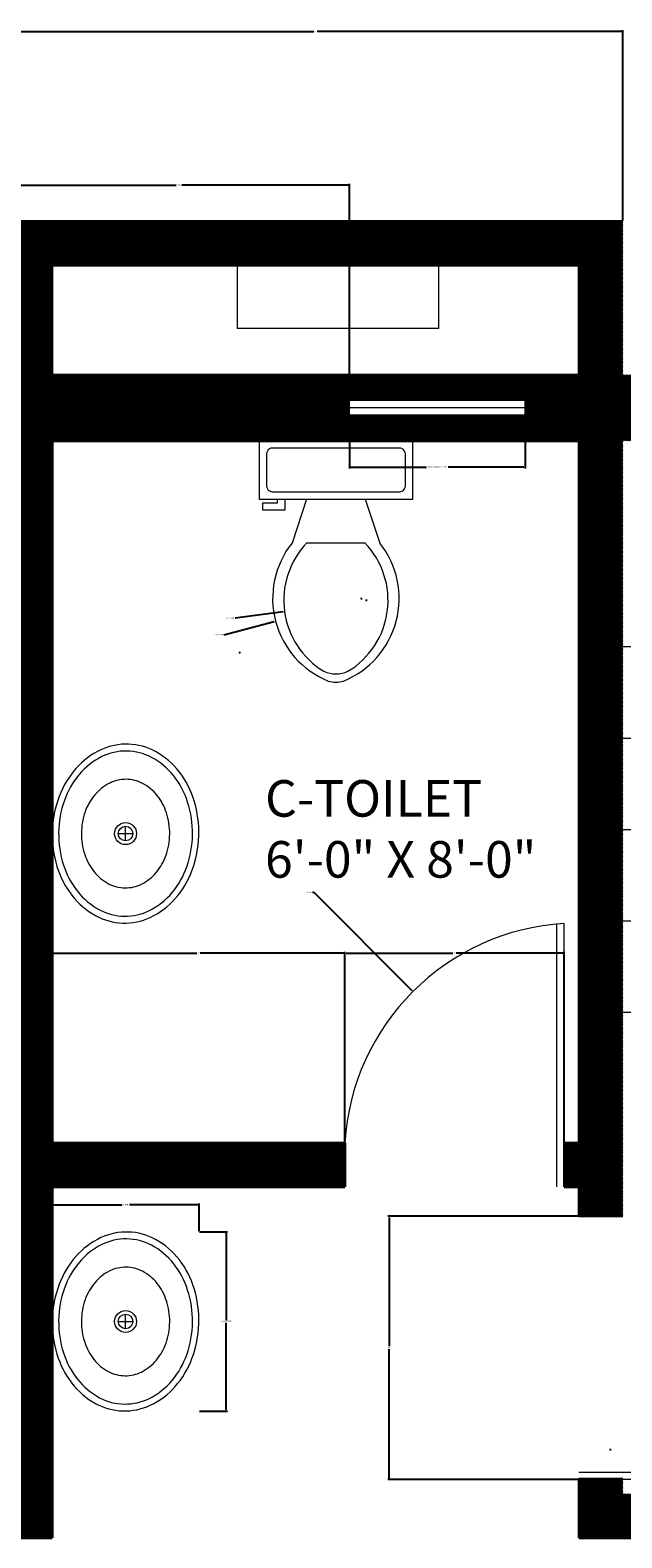
# Model space of a CAD drawing. Units: inches. Extents: x 557 to 1007, y 390 to 953.
# Tile 9 of 10: x 764 to 845, y 747 to 953. Entities that reach past the tile are written whole.
import ezdxf

# ---------------------------------------------------------------- set-up
doc = ezdxf.new("R2010")
doc.units = ezdxf.units.IN
doc.header["$LTSCALE"] = 5
doc.header["$MEASUREMENT"] = 0
for name, color, linetype, lineweight in [('A-ANNO-DIMS', 2, 'Continuous', 18), ('A-AREA-IDEN', 7, 'Continuous', 18), ('A-DOOR', 3, 'Continuous', 18), ('A-EQPM', 8, 'Continuous', 18), ('A-FLOR-FIXT', 9, 'Continuous', 18), ('A-FURN-PATT', 9, 'Continuous', 9), ('A-GLAZ', 4, 'Continuous', 18), ('A-WALL', 7, 'Continuous', 35)]:
    doc.layers.add(name, color=color, linetype=linetype, lineweight=lineweight)
doc.layers.add('A-GLAZ-PATT', color=141, linetype='Continuous', lineweight=9, true_color=0xadddf7)
doc.layers.add('A-WALL-PATT', color=251, linetype='Continuous', lineweight=9, true_color=0x636466)
doc.styles.get("Standard").update_dxf_attribs({"font": 'arial.ttf'})
doc.dimstyles.get("Standard").update_dxf_attribs({"dimtxt": 0.18, "dimasz": 0.18, "dimexe": 0.18, "dimexo": 0.0625, "dimgap": 0.09, "dimtad": 0, "dimtih": 1, "dimtoh": 1, "dimdec": 4, "dimzin": 0, "dimdsep": 46, "dimtxsty": 'Standard', "dimcen": 0.09, "dimadec": 0, "dimazin": 0, "dimtfac": 1, "dimtdec": 4, "dimtofl": 0, "dimtmove": 0, "dimatfit": 3, "dimfxl": 1, "dimtolj": 1, "dimtzin": 0, "dimarcsym": 0})

# ---------------------------------------------------------------- blocks, each defined once
blk = doc.blocks.new('Toilet - top')
for p, q in [((9.5, -6), (9.5, -2)), ((-8, -8.5), (-8, -8)), ((-7, -8), (-7, -9.5)), ((-4, -8), (-6, -14)), ((4, -8), (6, -14)), ((-10, -8.5), (-8, -8.5)), ((-10, -9.5), (-10, -8.5)), ((-7, -9.5), (-10, -9.5)), ((4, -14), (-4, -14))]:
    blk.add_line(p, q)
blk.add_lwpolyline([(10.5, -8), (10.5, 0), (-10.5, 0), (-10.5, -8)], close=True)
for points in [[(-9.5, -2), (-9.5, -6)], [(8.5, -1), (-8.5, -1)], [(-8.5, -7), (8.5, -7)]]:
    blk.add_lwpolyline(points)
for centre, radius, start, end in [((-8.62, -1.88), 0.884, 81.8699, 188.1301), ((8.62, -1.88), 0.884, 351.8699, 98.1301), ((-8.62, -6.12), 0.884, 171.8699, 278.1301), ((8.62, -6.12), 0.884, 261.8699, 8.1301), ((3.52, -21.58), 12.17, 141.4691, 247.9714), ((4.2, -21.82), 11.33, 136.3677, 238.9468), ((-3.52, -21.58), 12.17, 292.0284, 38.5307), ((-4.2, -21.82), 11.33, 301.053, 43.6321), ((0, -27.88), 4, 245.7318, 294.2682), ((0, -29), 4, 254.8605, 285.1395)]:
    blk.add_arc(centre, radius, start, end)
blk = doc.blocks.new('Sink - Oval top')
for p, q in [((-1, 0), (1, 0)), ((0, 1), (0, -1))]:
    blk.add_line(p, q)
for points in [[(-12.23, 0.39, 0.117634), (-11.46, -3.36, 0.104469), (-8.88, -6.8, 0.090016), (-5.08, -9.07, 0.08192), (-0.32, -10.02, 0.08192), (4.49, -9.38, 0.090016), (8.42, -7.36, 0.104469), (11.22, -4.09, 0.117634), (12.23, -0.39, 0.117634), (11.46, 3.36, 0.104469), (8.88, 6.8, 0.090016), (5.08, 9.07, 0.08192), (0.32, 10.02, 0.08192), (-4.49, 9.38, 0.090016), (-8.42, 7.36, 0.104469), (-11.22, 4.09, 0.117634)], [(-11.29, 0.16, 0.118622), (-10.52, -3.25, 0.104678), (-8.07, -6.36, 0.089562), (-4.54, -8.37, 0.081185), (-0.13, -9.15, 0.081185), (4.3, -8.49, 0.089562), (7.89, -6.58, 0.104678), (10.42, -3.55, 0.118622), (11.29, -0.16, 0.118622), (10.52, 3.25, 0.104678), (8.07, 6.36, 0.089562), (4.54, 8.37, 0.081185), (0.13, 9.15, 0.081185), (-4.3, 8.49, 0.089562), (-7.89, 6.58, 0.104678), (-10.42, 3.55, 0.118622)], [(-7.42, 0.08, 0.118283), (-6.91, -2.17, 0.104607), (-5.29, -4.21, 0.089718), (-2.97, -5.53, 0.081436), (-0.07, -6.04, 0.081436), (2.84, -5.59, 0.089718), (5.2, -4.33, 0.104607), (6.86, -2.32, 0.118283), (7.42, -0.08, 0.118283), (6.91, 2.17, 0.104607), (5.29, 4.21, 0.089718), (2.97, 5.53, 0.081436), (0.07, 6.04, 0.081436), (-2.84, 5.59, 0.089718), (-5.2, 4.33, 0.104607), (-6.86, 2.32, 0.118283)]]:
    blk.add_lwpolyline(points, format="xyb", close=True)
for radius in [1.5, 1]:
    blk.add_circle((0, 0), radius)
blk = doc.blocks.new('WIN-24-VENT')
for p, q in [((0, 0), (0, 9)), ((24, 0), (24, 9)), ((24, 5.5), (0, 5.5)), ((24, 4.5), (0, 4.5)), ((24, 3.5), (0, 3.5))]:
    blk.add_line(p, q)
blk = doc.blocks.new('*D27')
at = {"layer": 'A-ANNO-DIMS', "color": 0, "lineweight": -2, "ltscale": 5, "transparency": 16777216}
for p, q in [((787.56, 788.76), (791.36, 788.76)), ((791.18, 788.58), (791.18, 776.67)), ((791.18, 764.39), (791.18, 776.3)), ((787.56, 764.21), (791.36, 764.21))]:
    blk.add_line(p, q, dxfattribs=at)
at = {"layer": 'A-ANNO-DIMS', "color": 0, "ltscale": 5, "transparency": 16777216}
for points in [[(791.15, 788.58), (791.21, 788.58), (791.18, 788.76)], [(791.15, 764.39), (791.21, 764.39), (791.18, 764.21)]]:
    blk.add_solid(points, dxfattribs=at)
at = {"layer": 'Defpoints', "color": 0, "ltscale": 5, "transparency": 16777216}
for p in [(787.5, 788.76), (791.18, 788.76), (787.5, 764.21)]:
    blk.add_point(p, dxfattribs=at)
at = {"layer": 'A-ANNO-DIMS', "color": 0, "ltscale": 5, "transparency": 16777216, "insert": (791.18, 776.49), "char_height": 0.18, "attachment_point": 5}
blk.add_mtext('\\A1;BASIN 25 TYP.', dxfattribs=at)
blk = doc.blocks.new('*D28')
at = {"layer": 'A-ANNO-DIMS', "color": 0, "lineweight": -2, "ltscale": 5, "transparency": 16777216}
for p, q in [((767.36, 788.83), (767.36, 792.63)), ((767.54, 792.45), (776.9, 792.45)), ((787.32, 792.45), (777.96, 792.45)), ((787.5, 788.83), (787.5, 792.63))]:
    blk.add_line(p, q, dxfattribs=at)
at = {"layer": 'A-ANNO-DIMS', "color": 0, "ltscale": 5, "transparency": 16777216}
for points in [[(767.54, 792.48), (767.54, 792.42), (767.36, 792.45)], [(787.32, 792.48), (787.32, 792.42), (787.5, 792.45)]]:
    blk.add_solid(points, dxfattribs=at)
at = {"layer": 'Defpoints', "color": 0, "ltscale": 5, "transparency": 16777216}
for p in [(767.36, 792.45), (767.36, 788.76), (787.5, 788.76)]:
    blk.add_point(p, dxfattribs=at)
at = {"layer": 'A-ANNO-DIMS', "color": 0, "ltscale": 5, "transparency": 16777216, "insert": (777.43, 792.45), "char_height": 0.18, "attachment_point": 5}
blk.add_mtext('\\A1;20 TYP.', dxfattribs=at)
blk = doc.blocks.new('*D31')
at = {"layer": 'A-ANNO-DIMS', "color": 0, "lineweight": -2, "ltscale": 5, "transparency": 16777216}
for p, q in [((808.06, 896.84), (808.06, 893.12)), ((832.06, 896.84), (832.06, 893.12)), ((808.24, 893.3), (818.57, 893.3)), ((831.88, 893.3), (821.55, 893.3))]:
    blk.add_line(p, q, dxfattribs=at)
at = {"layer": 'A-ANNO-DIMS', "color": 0, "ltscale": 5, "transparency": 16777216}
for points in [[(808.24, 893.33), (808.24, 893.27), (808.06, 893.3)], [(831.88, 893.33), (831.88, 893.27), (832.06, 893.3)]]:
    blk.add_solid(points, dxfattribs=at)
at = {"layer": 'Defpoints', "color": 0, "ltscale": 5, "transparency": 16777216}
for p in [(808.06, 896.9), (832.06, 896.9), (832.06, 893.3)]:
    blk.add_point(p, dxfattribs=at)
at = {"layer": 'A-ANNO-DIMS', "color": 0, "ltscale": 5, "transparency": 16777216, "insert": (820.06, 893.3), "char_height": 0.18, "attachment_point": 5}
blk.add_mtext('\\A1;VENT WINDOW 24 TYP.', dxfattribs=at)
blk = doc.blocks.new('*D32')
at = {"layer": 'A-ANNO-DIMS', "color": 0, "lineweight": -2, "ltscale": 5, "transparency": 16777216}
for p, q in [((832.12, 905.9), (835.84, 905.9)), ((835.66, 905.72), (835.66, 901.59)), ((835.66, 897.08), (835.66, 901.22)), ((832.12, 896.9), (835.84, 896.9))]:
    blk.add_line(p, q, dxfattribs=at)
at = {"layer": 'A-ANNO-DIMS', "color": 0, "ltscale": 5, "transparency": 16777216}
for points in [[(835.63, 905.72), (835.69, 905.72), (835.66, 905.9)], [(835.63, 897.08), (835.69, 897.08), (835.66, 896.9)]]:
    blk.add_solid(points, dxfattribs=at)
at = {"layer": 'Defpoints', "color": 0, "ltscale": 5, "transparency": 16777216}
for p in [(832.06, 905.9), (835.66, 905.9), (832.06, 896.9)]:
    blk.add_point(p, dxfattribs=at)
at = {"layer": 'A-ANNO-DIMS', "color": 0, "ltscale": 5, "transparency": 16777216, "insert": (835.66, 901.4), "char_height": 0.18, "attachment_point": 5}
blk.add_mtext('\\A1;9 TYP.', dxfattribs=at)
blk = doc.blocks.new('*D46')
at = {"layer": 'A-ANNO-DIMS', "color": 0, "lineweight": -2, "ltscale": 5, "transparency": 16777216}
for p, q in [((761.34, 926.9), (556.69, 926.9)), ((556.87, 926.72), (556.87, 671.59)), ((556.87, 416.08), (556.87, 671.22)), ((773.34, 415.9), (556.69, 415.9))]:
    blk.add_line(p, q, dxfattribs=at)
at = {"layer": 'A-ANNO-DIMS', "color": 0, "ltscale": 5, "transparency": 16777216}
for points in [[(556.84, 926.72), (556.9, 926.72), (556.87, 926.9)], [(556.84, 416.08), (556.9, 416.08), (556.87, 415.9)]]:
    blk.add_solid(points, dxfattribs=at)
at = {"layer": 'Defpoints', "color": 0, "ltscale": 5, "transparency": 16777216}
for p in [(556.87, 926.9), (761.41, 926.9), (773.41, 415.9)]:
    blk.add_point(p, dxfattribs=at)
at = {"layer": 'A-ANNO-DIMS', "color": 0, "ltscale": 5, "transparency": 16777216, "insert": (556.87, 671.4), "char_height": 0.18, "attachment_point": 5}
blk.add_mtext('\\A1;511', dxfattribs=at)
blk = doc.blocks.new('*D50')
at = {"layer": 'A-ANNO-DIMS', "color": 0, "lineweight": -2, "ltscale": 5, "transparency": 16777216}
for p, q in [((761.41, 926.97), (761.41, 953.03)), ((761.59, 952.85), (803.19, 952.85)), ((845.23, 952.85), (803.62, 952.85)), ((845.41, 926.97), (845.41, 953.03))]:
    blk.add_line(p, q, dxfattribs=at)
at = {"layer": 'A-ANNO-DIMS', "color": 0, "ltscale": 5, "transparency": 16777216}
for points in [[(761.59, 952.88), (761.59, 952.82), (761.41, 952.85)], [(845.23, 952.88), (845.23, 952.82), (845.41, 952.85)]]:
    blk.add_solid(points, dxfattribs=at)
at = {"layer": 'Defpoints', "color": 0, "ltscale": 5, "transparency": 16777216}
for p in [(845.41, 952.85), (761.41, 926.9), (845.41, 926.9)]:
    blk.add_point(p, dxfattribs=at)
at = {"layer": 'A-ANNO-DIMS', "color": 0, "ltscale": 5, "transparency": 16777216, "insert": (803.41, 952.85), "char_height": 0.18, "attachment_point": 5}
blk.add_mtext('\\A1;84', dxfattribs=at)
blk = doc.blocks.new('*D70')
at = {"layer": 'A-ANNO-DIMS', "color": 0, "lineweight": -2, "ltscale": 5, "transparency": 16777216}
for p, q in [((807.41, 800.97), (807.41, 827.03)), ((807.59, 826.85), (822.19, 826.85)), ((837.23, 826.85), (822.62, 826.85)), ((837.41, 800.97), (837.41, 827.03))]:
    blk.add_line(p, q, dxfattribs=at)
at = {"layer": 'A-ANNO-DIMS', "color": 0, "ltscale": 5, "transparency": 16777216}
for points in [[(807.59, 826.88), (807.59, 826.82), (807.41, 826.85)], [(837.23, 826.88), (837.23, 826.82), (837.41, 826.85)]]:
    blk.add_solid(points, dxfattribs=at)
at = {"layer": 'Defpoints', "color": 0, "ltscale": 5, "transparency": 16777216}
for p in [(837.41, 826.85), (807.41, 800.9), (837.41, 800.9)]:
    blk.add_point(p, dxfattribs=at)
at = {"layer": 'A-ANNO-DIMS', "color": 0, "ltscale": 5, "transparency": 16777216, "insert": (822.41, 826.85), "char_height": 0.18, "attachment_point": 5}
blk.add_mtext('\\A1;30', dxfattribs=at)
blk = doc.blocks.new('*D71')
at = {"layer": 'A-ANNO-DIMS', "color": 0, "lineweight": -2, "ltscale": 5, "transparency": 16777216}
for p, q in [((839.34, 790.9), (813.28, 790.9)), ((813.46, 790.72), (813.46, 773.09)), ((813.46, 755.08), (813.46, 772.72)), ((839.34, 754.9), (813.28, 754.9))]:
    blk.add_line(p, q, dxfattribs=at)
at = {"layer": 'A-ANNO-DIMS', "color": 0, "ltscale": 5, "transparency": 16777216}
for points in [[(813.43, 790.72), (813.49, 790.72), (813.46, 790.9)], [(813.43, 755.08), (813.49, 755.08), (813.46, 754.9)]]:
    blk.add_solid(points, dxfattribs=at)
at = {"layer": 'Defpoints', "color": 0, "ltscale": 5, "transparency": 16777216}
for p in [(813.46, 790.9), (839.41, 790.9), (839.41, 754.9)]:
    blk.add_point(p, dxfattribs=at)
at = {"layer": 'A-ANNO-DIMS', "color": 0, "ltscale": 5, "transparency": 16777216, "insert": (813.46, 772.9), "char_height": 0.18, "attachment_point": 5}
blk.add_mtext('\\A1;36', dxfattribs=at)
blk = doc.blocks.new('*D76')
at = {"layer": 'A-ANNO-DIMS', "color": 0, "lineweight": -2, "ltscale": 5, "transparency": 16777216}
for p, q in [((761.41, 905.97), (761.41, 932.03)), ((761.59, 931.85), (784.34, 931.85)), ((807.88, 931.85), (785.13, 931.85)), ((808.06, 905.97), (808.06, 932.03))]:
    blk.add_line(p, q, dxfattribs=at)
at = {"layer": 'A-ANNO-DIMS', "color": 0, "ltscale": 5, "transparency": 16777216}
for points in [[(761.59, 931.88), (761.59, 931.82), (761.41, 931.85)], [(807.88, 931.88), (807.88, 931.82), (808.06, 931.85)]]:
    blk.add_solid(points, dxfattribs=at)
at = {"layer": 'Defpoints', "color": 0, "ltscale": 5, "transparency": 16777216}
for p in [(808.06, 931.85), (761.41, 905.9), (808.06, 905.9)]:
    blk.add_point(p, dxfattribs=at)
at = {"layer": 'A-ANNO-DIMS', "color": 0, "ltscale": 5, "transparency": 16777216, "insert": (784.73, 931.85), "char_height": 0.18, "attachment_point": 5}
blk.add_mtext('\\A1;46.66', dxfattribs=at)
blk = doc.blocks.new('*D99')
at = {"layer": 'A-ANNO-DIMS', "color": 0, "lineweight": -2, "ltscale": 5, "transparency": 16777216}
for p, q in [((767.41, 800.97), (767.41, 827.03)), ((767.59, 826.85), (787.18, 826.85)), ((807.23, 826.85), (787.63, 826.85)), ((807.41, 800.97), (807.41, 827.03))]:
    blk.add_line(p, q, dxfattribs=at)
at = {"layer": 'A-ANNO-DIMS', "color": 0, "ltscale": 5, "transparency": 16777216}
for points in [[(767.59, 826.88), (767.59, 826.82), (767.41, 826.85)], [(807.23, 826.88), (807.23, 826.82), (807.41, 826.85)]]:
    blk.add_solid(points, dxfattribs=at)
at = {"layer": 'Defpoints', "color": 0, "ltscale": 5, "transparency": 16777216}
for p in [(807.41, 826.85), (767.41, 800.9), (807.41, 800.9)]:
    blk.add_point(p, dxfattribs=at)
at = {"layer": 'A-ANNO-DIMS', "color": 0, "ltscale": 5, "transparency": 16777216, "insert": (787.41, 826.85), "char_height": 0.18, "attachment_point": 5}
blk.add_mtext('\\A1;40', dxfattribs=at)
blk = doc.blocks.new('*D107')
at = {"layer": 'A-ANNO-DIMS', "color": 0, "lineweight": -2, "ltscale": 5, "transparency": 16777216}
for p, q in [((802.97, 835.16), (803.15, 835.16)), ((803.15, 835.16), (816.59, 821.72)), ((839.23, 798.99), (839.41, 798.99)), ((839.32, 798.9), (839.32, 799.08))]:
    blk.add_line(p, q, dxfattribs=at)
at = {"layer": 'A-ANNO-DIMS', "color": 0, "ltscale": 5, "transparency": 16777216}
blk.add_solid([(816.61, 821.74), (816.56, 821.7), (816.71, 821.6)], dxfattribs=at)
at = {"layer": 'Defpoints', "color": 0, "ltscale": 5, "transparency": 16777216}
for p in [(816.71, 821.6), (839.32, 798.99)]:
    blk.add_point(p, dxfattribs=at)
at = {"layer": 'A-ANNO-DIMS', "color": 0, "ltscale": 5, "transparency": 16777216, "insert": (802.49, 835.16), "char_height": 0.18, "attachment_point": 5}
blk.add_mtext('\\A1;R31.98', dxfattribs=at)
blk = doc.blocks.new('*D108')
at = {"layer": 'A-ANNO-DIMS', "color": 0, "lineweight": -2, "ltscale": 5, "transparency": 16777216}
for p, q in [((882.99, 791.73), (868.4, 779.57)), ((883.17, 791.73), (882.99, 791.73)), ((843.63, 759), (843.81, 759)), ((843.72, 758.91), (843.72, 759.09))]:
    blk.add_line(p, q, dxfattribs=at)
at = {"layer": 'A-ANNO-DIMS', "color": 0, "ltscale": 5, "transparency": 16777216}
blk.add_solid([(868.38, 779.59), (868.42, 779.55), (868.26, 779.45)], dxfattribs=at)
at = {"layer": 'Defpoints', "color": 0, "ltscale": 5, "transparency": 16777216}
for p in [(868.26, 779.45), (843.72, 759)]:
    blk.add_point(p, dxfattribs=at)
at = {"layer": 'A-ANNO-DIMS', "color": 0, "ltscale": 5, "transparency": 16777216, "insert": (883.65, 791.73), "char_height": 0.18, "attachment_point": 5}
blk.add_mtext('\\A1;R31.95', dxfattribs=at)
blk = doc.blocks.new('*D112')
at = {"layer": 'A-ANNO-DIMS', "color": 0, "lineweight": -2, "ltscale": 5, "transparency": 16777216}
for p, q in [((792.94, 867.96), (793.12, 867.96)), ((793.03, 867.87), (793.03, 868.05)), ((690.71, 858.03), (728.9, 861.74))]:
    blk.add_line(p, q, dxfattribs=at)
at = {"layer": 'A-ANNO-DIMS', "color": 0, "ltscale": 5, "transparency": 16777216}
blk.add_solid([(728.9, 861.77), (728.91, 861.71), (729.08, 861.76)], dxfattribs=at)
at = {"layer": 'Defpoints', "color": 0, "ltscale": 5, "transparency": 16777216}
for p in [(793.03, 867.96), (729.08, 861.76)]:
    blk.add_point(p, dxfattribs=at)
at = {"layer": 'A-ANNO-DIMS', "color": 0, "ltscale": 5, "transparency": 16777216, "insert": (690.03, 858.03), "char_height": 0.18, "attachment_point": 5}
blk.add_mtext('\\A1;4X R64.25', dxfattribs=at)
blk = doc.blocks.new('*D116')
at = {"layer": 'A-ANNO-DIMS', "color": 0, "lineweight": -2, "ltscale": 5, "transparency": 16777216}
for p, q in [((809.62, 875.32), (809.8, 875.32)), ((809.71, 875.23), (809.71, 875.41)), ((790.88, 870.38), (797.76, 872.19))]:
    blk.add_line(p, q, dxfattribs=at)
at = {"layer": 'A-ANNO-DIMS', "color": 0, "ltscale": 5, "transparency": 16777216}
blk.add_solid([(797.76, 872.22), (797.77, 872.16), (797.94, 872.23)], dxfattribs=at)
at = {"layer": 'Defpoints', "color": 0, "ltscale": 5, "transparency": 16777216}
for p in [(809.71, 875.32), (797.94, 872.23)]:
    blk.add_point(p, dxfattribs=at)
at = {"layer": 'A-ANNO-DIMS', "color": 0, "ltscale": 5, "transparency": 16777216, "insert": (790.2, 870.38), "char_height": 0.18, "attachment_point": 5}
blk.add_mtext('\\A1;4X R12.17', dxfattribs=at)
blk = doc.blocks.new('*D117')
at = {"layer": 'A-ANNO-DIMS', "color": 0, "lineweight": -2, "ltscale": 5, "transparency": 16777216}
for p, q in [((810.3, 875.09), (810.48, 875.09)), ((810.39, 875), (810.39, 875.18)), ((792.42, 872.67), (798.98, 873.55))]:
    blk.add_line(p, q, dxfattribs=at)
at = {"layer": 'A-ANNO-DIMS', "color": 0, "ltscale": 5, "transparency": 16777216}
blk.add_solid([(798.98, 873.58), (798.99, 873.52), (799.16, 873.58)], dxfattribs=at)
at = {"layer": 'Defpoints', "color": 0, "ltscale": 5, "transparency": 16777216}
for p in [(810.39, 875.09), (799.16, 873.58)]:
    blk.add_point(p, dxfattribs=at)
at = {"layer": 'A-ANNO-DIMS', "color": 0, "ltscale": 5, "transparency": 16777216, "insert": (791.75, 872.67), "char_height": 0.18, "attachment_point": 5}
blk.add_mtext('\\A1;4X R11.33', dxfattribs=at)

msp = doc.modelspace()

# ---------------------------------------------------------------- hatches: boundary and pattern name
at = {"layer": 'A-FURN-PATT', "ltscale": 5}
h = msp.add_hatch(dxfattribs=at)
h.set_pattern_fill('GRAVEL', color=256, scale=25)
h.set_pattern_definition([(228.01279, (18, 25), (-200, -225), [3.3634, -332.9772]), (184.96974, (15.75, 22.5), (300, 25), [5.7717, -571.39812]), (132.51045, (10, 22), (250, -275), [4.0697, -402.9008]), (267.27369, (0.25, 15.75), (25, 500), [5.25595, -520.33895]), (292.83365, (0, 10.5), (-125, 300), [5.15387, -510.23433]), (357.27369, (2, 5.75), (-500, 25), [5.25595, -520.33895]), (37.69424, (7.25, 5.5), (-325, -250), [6.95072, -688.1212]), (72.25533, (12.75, 9.75), (175, 550), [6.5622, -649.65804]), (121.42957, (14.75, 16), (-200, 325), [5.27375, -522.10183]), (175.23636, (12, 20.5), (275, -25), [6.0208, -295.01906]), (222.39744, (6, 21), (-300, -275), [7.7862, -770.83438]), (138.81407, (25, 15.5), (-175, 150), [2.65752, -263.0961]), (171.46923, (23, 17.25), (325, -50), [5.05593, -500.5378]), (225, (18, 18), (-3e-15, -25), [3.53552, -31.8198]), (203.1986, (16.25, 21), (125, 50), [1.90395, -188.49038]), (291.8014, (14.5, 20.25), (-25, 75), [2.69257, -131.93655]), (30.96376, (15.5, 17.75), (75, 50), [4.37322, -141.40057]), (161.56505, (19.25, 20), (50, -25), [3.16228, -75.89467]), (16.38954, (0, 20.25), (250, 75), [4.43, -438.57113]), (70.34618, (4.25, 21.5), (-100, -275), [3.71652, -367.9352]), (293.1986, (19.25, 25), (-50, 125), [3.80788, -186.58645]), (343.61046, (20.75, 21.5), (-250, 75), [4.43, -438.57113]), (339.44395, (0, 4.75), (-125, 50), [4.272, -209.3281]), (294.77514, (4, 3.25), (-125, 275), [3.57945, -354.36608]), (66.8014, (19.5, 0), (50, 125), [3.80788, -186.58645]), (17.35402, (21, 3.5), (-325, -100), [4.19078, -414.8856]), (69.44395, (7.25, 0), (-50, -125), [2.136, -211.4641]), (101.30993, (18, 0), (-25, 100), [1.27475, -126.20074]), (165.96376, (17.75, 1.25), (75, -25), [5.15388, -97.92377]), (186.00901, (12.75, 2.5), (250, 25), [4.77625, -472.84808]), (303.69007, (15.5, 15.5), (-25, 50), [3.60555, -86.53323]), (353.15723, (17.5, 12.5), (425, -50), [6.29485, -623.18907]), (60.9454, (23.75, 11.75), (-100, -175), [2.5739, -254.81685]), (90, (25, 14), (-25, 25), [1.5, -23.5]), (120.25644, (12.25, 3.25), (100, -175), [3.4731, -343.838]), (48.01279, (10.5, 6.25), (200, 225), [6.7268, -329.6138]), (0, (15, 11.25), (25, 25), [6.5, -18.5]), (325.30485, (21.5, 11.25), (250, -175), [3.95285, -391.33186]), (254.0546, (24.75, 9), (-25, -100), [3.64005, -178.3627]), (207.64598, (23.75, 5.5), (-475, -250), [5.92662, -586.73685]), (175.42608, (18.5, 2.75), (-325, 25), [6.26997, -620.72684])])
h.paths.add_polyline_path([(615.2525, 688.5, 1), (640.7475, 688.5, 1)])
h.paths.add_polyline_path([(917.0544, 663.8414, 0.33333323), (915.2241, 665.6717), (882.2793, 665.6717, 0.33333323), (880.449, 663.8414), (880.449, 649.1992, 0.33333323), (882.2793, 647.369), (915.2241, 647.369, 0.33333323), (917.0544, 649.1992)])
h.paths.add_polyline_path([(828.0807, 699.7098), (756.0807, 699.7098), (756.0807, 663.7098), (828.0807, 663.7098)])
h.paths.add_polyline_path([(787.5651, 663.7098), (768.5964, 663.7098), (769.8463, 655.7098), (786.3151, 655.7098)])
h.paths.add_polyline_path([(815.5651, 663.7098), (796.5964, 663.7098), (797.8463, 655.7098), (814.3151, 655.7098)])
h.paths.add_polyline_path([(836.0807, 689.9442), (828.0807, 691.1942), (828.0807, 672.2255), (836.0807, 673.4755)])
h.paths.add_polyline_path([(756.0807, 691.1942), (748.0807, 689.9442), (748.0807, 673.4755), (756.0807, 672.2255)])
h.paths.add_polyline_path([(786.3151, 707.7098), (769.8463, 707.7098), (768.5964, 699.7098), (787.5651, 699.7098)])
h.paths.add_polyline_path([(814.3151, 707.7098), (797.8463, 707.7098), (796.5964, 699.7098), (815.5651, 699.7098)])
h.paths.add_polyline_path([(917.4362, 607.3575), (889.5896, 607.3575), (889.5896, 586.4726), (917.4362, 586.4726)])
h.paths.add_polyline_path([(721.4053, 881.8539), (671.0053, 881.8539), (671.0053, 866.6539), (658.2053, 866.6539), (658.2053, 821.8539), (721.4053, 821.8539)])
h.paths.add_polyline_path([(925.4053, 875.1046), (875.0053, 875.1046), (875.0053, 859.9046), (862.2053, 859.9046), (862.2053, 815.1046), (925.4053, 815.1046)])
h.paths.add_polyline_path([(721.4053, 558.9046), (671.0053, 558.9046), (671.0053, 543.7046), (658.2053, 543.7046), (658.2053, 498.9046), (721.4053, 498.9046)])
at = {"layer": 'A-FURN-PATT'}
h = msp.add_hatch(dxfattribs=at)
h.set_pattern_fill('CROSS', color=256, scale=25)
h.paths.add_polyline_path([(925.4053, 875.1046), (875.0053, 875.1046), (875.0053, 859.9046), (862.2053, 859.9046), (862.2053, 815.1046), (925.4053, 815.1046)])
h.paths.add_polyline_path([(721.4053, 881.8539), (671.0053, 881.8539), (671.0053, 866.6539), (658.2053, 866.6539), (658.2053, 821.8539), (721.4053, 821.8539)])
h.paths.add_polyline_path([(671.0053, 881.8539), (655.8053, 866.6539), (671.0053, 866.6539)], flags=17)
h.paths.add_polyline_path([(671.0053, 881.8539), (641.4053, 881.8539), (641.4053, 821.8539), (655.8053, 821.8539), (655.8053, 829.8539), (642.6053, 829.8539), (642.6053, 850.6539), (655.8053, 850.6539), (655.8053, 853.0539), (642.6053, 853.0539), (642.6053, 873.8539), (657.8053, 873.8539), (657.8053, 868.6539)])
h.paths.add_polyline_path([(875.0053, 875.1046), (859.8053, 859.9046), (875.0053, 859.9046)], flags=17)
h.paths.add_polyline_path([(875.0053, 875.1046), (845.4053, 875.1046), (845.4053, 815.1046), (859.8053, 815.1046), (859.8053, 823.1046), (846.6053, 823.1046), (846.6053, 843.9046), (859.8053, 843.9046), (859.8053, 846.3046), (846.6053, 846.3046), (846.6053, 867.1046), (861.8053, 867.1046), (861.8053, 861.9046)])
h.paths.add_polyline_path([(721.4053, 558.9046), (671.0053, 558.9046), (671.0053, 543.7046), (658.2053, 543.7046), (658.2053, 498.9046), (721.4053, 498.9046)])
h.paths.add_polyline_path([(671.0053, 558.9046), (641.4053, 558.9046), (641.4053, 498.9046), (655.8053, 498.9046), (655.8053, 506.9046), (642.6053, 506.9046), (642.6053, 527.7046), (655.8053, 527.7046), (655.8053, 530.1046), (642.6053, 530.1046), (642.6053, 550.9046), (657.8053, 550.9046), (657.8053, 545.7046)])
h.paths.add_polyline_path([(671.0053, 558.9046), (657.8053, 545.7046), (655.8053, 543.7046), (671.0053, 543.7046)], flags=17)
h.paths.add_polyline_path([(873.1461, 661.8773, 0.41421356), (868.1461, 666.8773, -0.12244426), (867.1516, 666.8773), (855.014, 666.8773), (855.014, 647.2429), (867.4581, 647.2429, -0.08537395), (868.1461, 647.2429, 0.41421356), (873.1461, 652.2429)])
h.paths.add_polyline_path([(917.0544, 663.8414, 0.33333323), (915.2241, 665.6717), (882.2793, 665.6717, 0.33333323), (880.449, 663.8414), (880.449, 649.1992, 0.33333323), (882.2793, 647.369), (915.2241, 647.369, 0.33333323), (917.0544, 649.1992)])
h.paths.add_polyline_path([(944.9465, 667.5202), (932.6561, 667.5202, -0.10407786), (931.8144, 667.5202, 0.41421356), (926.8144, 662.5202), (926.8144, 652.8858, 0.41421356), (931.8144, 647.8858, -0.05611627), (932.2647, 647.8858), (944.9465, 647.8858)])
h.paths.add_polyline_path([(928.8341, 635.542, 0.41421356), (923.8341, 640.542), (914.1997, 640.542, 0.41421356), (909.1997, 635.542), (909.1997, 622.4099), (923.8341, 622.4099, 0.41421356), (928.8341, 627.4099)])
h.paths.add_polyline_path([(909.1997, 635.542, 0.41421356), (904.1997, 640.542), (894.5653, 640.542, 0.41421356), (889.5653, 635.542), (889.5653, 622.4099), (909.1997, 622.4099)])
h.paths.add_polyline_path([(889.5653, 635.542, 0.41421356), (884.5653, 640.542), (874.9308, 640.542, 0.41421356), (869.9308, 635.542), (869.9308, 627.4099, 0.41421356), (874.9308, 622.4099), (889.5653, 622.4099)])
at = {"layer": 'A-GLAZ-PATT'}
h = msp.add_hatch(dxfattribs=at)
h.set_pattern_fill('ANSI31', color=256)
h.paths.add_polyline_path([(635.9053, 814.7688), (636.9053, 814.7688), (636.9053, 838.7688), (632.4053, 838.7688), (632.4053, 790.7688), (635.9053, 790.7688)])
h.paths.add_polyline_path([(641.4053, 838.7688), (637.9053, 838.7688), (637.9053, 814.7688), (636.9053, 814.7688), (636.9053, 790.7688), (641.4053, 790.7688)])
h.paths.add_polyline_path([(603.4053, 728.9046, -0.41421356), (623.4053, 748.9046), (632.4053, 748.9046), (632.4053, 752.9046), (623.4053, 752.9046, 0.41421356), (599.4053, 728.9046), (599.4053, 614.9046), (603.4053, 614.9046)])
h.paths.add_polyline_path([(632.4053, 743.9046), (632.4053, 747.9046), (623.4053, 747.9046, 0.41421356), (604.4053, 728.9046), (604.4053, 614.9046), (608.4053, 614.9046), (608.4053, 719.9046, -0.41421356)])
h.paths.add_polyline_path([(683.4053, 722.9046), (678.9053, 722.9046), (678.9053, 698.9046), (679.9053, 698.9046), (679.9053, 662.9046), (678.9053, 662.9046), (678.9053, 638.9046), (683.4053, 638.9046)])
h.paths.add_polyline_path([(678.9053, 698.9046), (677.9053, 698.9046), (677.9053, 722.9046), (674.4053, 722.9046), (674.4053, 638.9046), (677.9053, 638.9046), (677.9053, 662.9046), (678.9053, 662.9046)])
h.paths.add_polyline_path([(635.9053, 593.9046), (632.4053, 593.9046), (632.4053, 557.9046), (635.9053, 557.9046)])
h.paths.add_polyline_path([(641.4053, 593.9046), (637.9053, 593.9046), (637.9053, 557.9046), (641.4053, 557.9046)])
h.paths.add_polyline_path([(764.9579, 448.9046), (716.9579, 448.9046), (716.9579, 445.4046), (740.9579, 445.4046), (740.9579, 444.4046), (764.9579, 444.4046)])
h.paths.add_polyline_path([(764.9579, 443.4046), (740.9579, 443.4046), (740.9579, 444.4046), (716.9579, 444.4046), (716.9579, 439.9046), (764.9579, 439.9046)])
h.paths.add_polyline_path([(938.4053, 905.9046), (878.4053, 905.9046), (878.4053, 902.4046), (908.4053, 902.4046), (908.4053, 901.4046), (938.4053, 901.4046)])
h.paths.add_polyline_path([(938.4053, 900.4046), (908.4053, 900.4046), (908.4053, 901.4046), (878.4053, 901.4046), (878.4053, 896.9046), (938.4053, 896.9046)])
h.paths.add_polyline_path([(724.9087, 905.9046), (676.9087, 905.9046), (676.9087, 902.4046), (701.4053, 902.4046), (701.4053, 901.4046), (724.9087, 901.4046)])
h.paths.add_polyline_path([(724.9087, 900.4046), (701.4053, 900.4046), (701.4053, 901.4046), (676.9087, 901.4046), (676.9087, 896.9046), (724.9087, 896.9046)])
h.paths.add_polyline_path([(832.0625, 905.9046), (808.0625, 905.9046), (808.0625, 902.4046), (832.0625, 902.4046)])
h.paths.add_polyline_path([(832.0625, 900.4046), (808.0625, 900.4046), (808.0625, 896.9046), (832.0625, 896.9046)])
at = {"layer": 'A-WALL-PATT'}
h = msp.add_hatch(dxfattribs=at)
h.set_pattern_fill('ANSI31', color=256)
h.paths.add_polyline_path([(808.0625, 905.9046), (767.4053, 905.9046), (767.4053, 920.9046), (839.4053, 920.9046), (839.4053, 905.9046), (832.0625, 905.9046), (832.0625, 896.9046), (839.4053, 896.9046), (839.4053, 800.9046), (837.4053, 800.9046), (837.4053, 794.9046), (839.4053, 794.9046), (839.4053, 790.9046), (845.4053, 790.9046), (845.4053, 896.9046), (878.4053, 896.9046), (878.4053, 905.9046), (845.4053, 905.9046), (845.4053, 926.9046), (761.4053, 926.9046), (761.4053, 914.9046), (761.4053, 905.9046), (724.9087, 905.9046), (724.9087, 896.9046), (761.4053, 896.9046), (761.4053, 752.9046), (759.4053, 752.9046), (759.4053, 746.9046), (767.4053, 746.9046), (767.4053, 794.9046), (807.4053, 794.9046), (807.4053, 800.9046), (767.4053, 800.9046), (767.4053, 896.9046), (808.0625, 896.9046)])
h.paths.add_polyline_path([(676.9087, 905.9046), (632.4053, 905.9046), (632.4053, 838.7688), (641.4053, 838.7688), (641.4053, 881.8539), (641.4053, 896.9046), (676.9087, 896.9046)])
h.paths.add_polyline_path([(980.4053, 905.9046), (938.4053, 905.9046), (938.4053, 896.9046), (971.4053, 896.9046), (971.4053, 752.9046), (845.4053, 752.9046), (845.4053, 754.9046), (839.4053, 754.9046), (839.4053, 746.9046), (971.4053, 746.9046), (971.4053, 720.1788), (980.4053, 720.1788)])
h.paths.add_polyline_path([(723.4053, 752.9046), (641.4053, 752.9046), (641.4053, 790.7688), (632.4053, 790.7688), (632.4053, 743.9046), (674.4053, 743.9046), (674.4053, 722.9046), (683.4053, 722.9046), (683.4053, 746.9046), (723.4053, 746.9046)])
h.paths.add_polyline_path([(980.4053, 684.1788), (971.4053, 684.1788), (971.4053, 614.9046), (845.4053, 614.9046), (845.4053, 608.9046), (971.4053, 608.9046), (971.4053, 512.9046), (908.7697, 512.9046), (908.7697, 508.9046), (971.4053, 508.9046), (971.4053, 448.9046), (845.4053, 448.9046), (845.4053, 508.9046), (878.7697, 508.9046), (878.7697, 512.9046), (845.4053, 512.9046), (845.4053, 562.9046), (779.4053, 562.9046), (779.4053, 614.9046), (761.4053, 614.9046), (761.4053, 608.9046), (773.4053, 608.9046), (773.4053, 512.636), (779.4053, 512.636), (779.4053, 556.9046), (839.4053, 556.9046), (839.4053, 448.9046), (830.432, 448.9046), (830.432, 439.9046), (839.4053, 439.9046), (839.4053, 433.0506), (839.4053, 421.9046), (779.4053, 421.9046), (779.4053, 439.9046), (796.9656, 439.9046), (806.432, 439.9046), (806.432, 448.9046), (779.4053, 448.9046), (779.4053, 482.636), (773.4053, 482.636), (773.4053, 448.9046), (764.9579, 448.9046), (764.9579, 439.9046), (773.4053, 439.9046), (773.4053, 415.9046), (845.4053, 415.9046), (845.4053, 439.9046), (980.4053, 439.9046)])
h.paths.add_polyline_path([(716.9579, 448.9046), (641.4053, 448.9046), (641.4053, 557.9046), (632.4053, 557.9046), (632.4053, 439.9046), (716.9579, 439.9046)])
h.paths.add_polyline_path([(725.4053, 614.9046), (683.4053, 614.9046), (683.4053, 638.9046), (674.4053, 638.9046), (674.4053, 614.9046), (608.4053, 614.9046), (582.8236, 614.9046), (582.8236, 605.9046), (599.4053, 605.9046), (632.4053, 605.9046), (641.4053, 605.9046), (641.4053, 608.9046), (725.4053, 608.9046)])
h.paths.add_polyline_path([(641.4053, 605.9046), (632.4053, 605.9046), (632.4053, 593.9046), (641.4053, 593.9046)])

# ---------------------------------------------------------------- linework, layer by layer
at = {"layer": 'A-DOOR'}
for p, q in [((836.4053, 794.9046), (836.4053, 830.9046)), ((837.4053, 794.9046), (837.4053, 830.9046)), ((839.4053, 755.9046), (875.4053, 755.9046)), ((839.4053, 754.9046), (875.4053, 754.9046))]:
    msp.add_line(p, q, dxfattribs=at)
msp.add_arc((839.3247, 798.9851), 31.9771, 93.441298, 176.558702, dxfattribs=at)
at = {"layer": 'A-EQPM'}
msp.add_lwpolyline([(792.7298, 920.9046), (820.2211, 920.9046), (820.2211, 912.2341), (792.7298, 912.2341)], close=True, dxfattribs=at)
at = {"layer": 'A-WALL'}
for p, q in [((761.4053, 926.9046), (845.4053, 926.9046)), ((767.4053, 905.9046), (767.4053, 920.9046)), ((767.4053, 920.9046), (839.4053, 920.9046)), ((839.4053, 920.9046), (839.4053, 905.9046)), ((767.4053, 905.9046), (839.4053, 905.9046)), ((767.4053, 896.9046), (767.4053, 800.9046)), ((767.4053, 896.9046), (839.4053, 896.9046)), ((839.4053, 896.9046), (839.4053, 800.9046)), ((767.4053, 800.9046), (807.4053, 800.9046)), ((807.4053, 800.9046), (807.4053, 794.9046)), ((837.4053, 800.9046), (837.4053, 794.9046)), ((837.4053, 800.9046), (839.4053, 800.9046)), ((767.4053, 794.9046), (807.4053, 794.9046)), ((767.4053, 794.9046), (767.4053, 746.9046)), ((837.4053, 794.9046), (839.4053, 794.9046)), ((839.4053, 794.9046), (839.4053, 790.9046)), ((845.4053, 790.9046), (839.4053, 790.9046)), ((845.4053, 754.9046), (839.4053, 754.9046)), ((839.4053, 754.9046), (839.4053, 746.9046)), ((759.4053, 746.9046), (767.4053, 746.9046)), ((839.4053, 746.9046), (971.4053, 746.9046))]:
    msp.add_line(p, q, dxfattribs=at)

# ---------------------------------------------------------------- block references
at = {"layer": 'A-FLOR-FIXT'}
msp.add_blockref('Toilet - top', (806.1881, 896.9046), dxfattribs=at)
at = {"layer": 'A-FLOR-FIXT', "rotation": 90}
for p in [(777.4288, 843.19), (777.4288, 776.4875)]:
    msp.add_blockref('Sink - Oval top', p, dxfattribs=at)
at = {"layer": 'A-GLAZ'}
msp.add_blockref('WIN-24-VENT', (808.062, 896.905), dxfattribs=at)

# ---------------------------------------------------------------- texts
at = {"layer": 'A-AREA-IDEN', "insert": (796.5, 850.5), "char_height": 5, "attachment_point": 1}
msp.add_mtext_dynamic_manual_height_columns('C-TOILET\\P6\'-0" X 8\'-0"', width=125, gutter_width=1, heights=[0], dxfattribs=at)

# ---------------------------------------------------------------- dimensions: what is measured, and where the dimension line sits
at = {"layer": 'A-ANNO-DIMS', "ltscale": 5}
for base, p1, p2, picture, middle in [((845.4053, 952.8546), (761.4053, 926.9046), (845.4053, 926.9046), '*D50', (803.4053, 952.8546)), ((837.4053, 826.8546), (807.4053, 800.9046), (837.4053, 800.9046), '*D70', (822.4053, 826.8546))]:
    dim = msp.add_linear_dim(base=base, p1=p1, p2=p2, dimstyle='Standard', override={"dimdec": 0, "dimlfac": 1, "dimrnd": 0, "dimzin": 0, "dimdsep": 46, "dimlunit": 2}, dxfattribs=at)
    dim.commit()
    dim.dimension.update_dxf_attribs({"geometry": picture, "text_midpoint": middle})
for base, p1, p2, angle, override, picture, middle in [((808.0625, 931.8546), (761.4053, 905.9046), (808.0625, 905.9046), 0, {"dimdec": 2, "dimlfac": 1, "dimrnd": 0, "dimzin": 0, "dimdsep": 46, "dimlunit": 2}, '*D76', (784.7339, 931.8546)), ((556.8736, 926.9046), (773.4053, 415.9046), (761.4053, 926.9046), 90, {"dimdec": 0, "dimlfac": 1, "dimrnd": 0, "dimzin": 0, "dimdsep": 46, "dimlunit": 2}, '*D46', (556.8736, 671.4046)), ((807.4053, 826.8546), (767.4053, 800.9046), (807.4053, 800.9046), 0, {"dimdec": 0, "dimlfac": 1, "dimrnd": 0, "dimzin": 0, "dimdsep": 46, "dimlunit": 2}, '*D99', (787.4053, 826.8546)), ((813.4553, 790.9046), (839.4053, 754.9046), (839.4053, 790.9046), 90, {"dimdec": 0, "dimlfac": 1, "dimrnd": 0, "dimzin": 0, "dimdsep": 46, "dimlunit": 2}, '*D71', (813.4553, 772.9046))]:
    dim = msp.add_linear_dim(base=base, p1=p1, p2=p2, angle=angle, dimstyle='Standard', override=override, dxfattribs=at)
    dim.commit()
    dim.dimension.update_dxf_attribs({"geometry": picture, "text_midpoint": middle})
for base, p1, p2, angle, text, picture, middle in [((835.6625, 905.9046), (832.0625, 896.9046), (832.0625, 905.9046), 90, '<> TYP.', '*D32', (835.6625, 901.4046)), ((767.3606, 792.4456), (787.4971, 788.7629), (767.3606, 788.7629), 180, '<> TYP.', '*D28', (777.4288, 792.4456)), ((791.1798, 788.7629), (787.4971, 764.2121), (787.4971, 788.7629), 90, 'BASIN <> TYP.', '*D27', (791.1798, 776.4875))]:
    dim = msp.add_linear_dim(base=base, p1=p1, p2=p2, angle=angle, text=text, dimstyle='Standard', override={"dimdec": 0, "dimlfac": 1, "dimrnd": 0, "dimzin": 0, "dimdsep": 46, "dimlunit": 2}, dxfattribs=at)
    dim.commit()
    dim.dimension.update_dxf_attribs({"geometry": picture, "text_midpoint": middle})
dim = msp.add_linear_dim(base=(832.0625, 893.3046), p1=(808.0625, 896.9046), p2=(832.0625, 896.9046), text='VENT WINDOW <> TYP.', dimstyle='Standard', override={"dimdec": 0, "dimlfac": 1, "dimrnd": 0, "dimzin": 0, "dimdsep": 46, "dimlunit": 2}, dxfattribs=at)
dim.commit()
dim.dimension.update_dxf_attribs({"geometry": '*D31', "text_midpoint": (820.0625, 893.3046)})
for center, mpoint, picture, middle in [((809.7077, 875.3241), (797.9381, 872.232), '*D116', (790.8763, 870.3768)), ((810.3881, 875.0872), (799.1599, 873.578), '*D117', (792.4229, 872.6725)), ((793.0326, 867.9551), (729.0824, 861.755), '*D112', (690.7124, 858.035))]:
    dim = msp.add_radius_dim(center=center, mpoint=mpoint, text='4X <>', dimstyle='Standard', override={"dimdec": 2, "dimlfac": 1, "dimrnd": 0, "dimzin": 0, "dimdsep": 46, "dimlunit": 2}, dxfattribs=at)
    dim.commit()
    dim.dimension.update_dxf_attribs({"geometry": picture, "text_midpoint": middle, "dimtype": 164})
for center, mpoint, picture, middle in [((839.3247, 798.9851), (816.7131, 821.5959), '*D107', (802.4861, 835.1624)), ((843.7185, 758.999), (868.2632, 779.4531), '*D108', (883.6505, 791.7256))]:
    dim = msp.add_radius_dim(center=center, mpoint=mpoint, dimstyle='Standard', override={"dimdec": 2, "dimlfac": 1, "dimrnd": 0, "dimzin": 0, "dimdsep": 46, "dimlunit": 2}, dxfattribs=at)
    dim.commit()
    dim.dimension.update_dxf_attribs({"geometry": picture, "text_midpoint": middle, "dimtype": 164})

doc.saveas('drawing.dxf')
